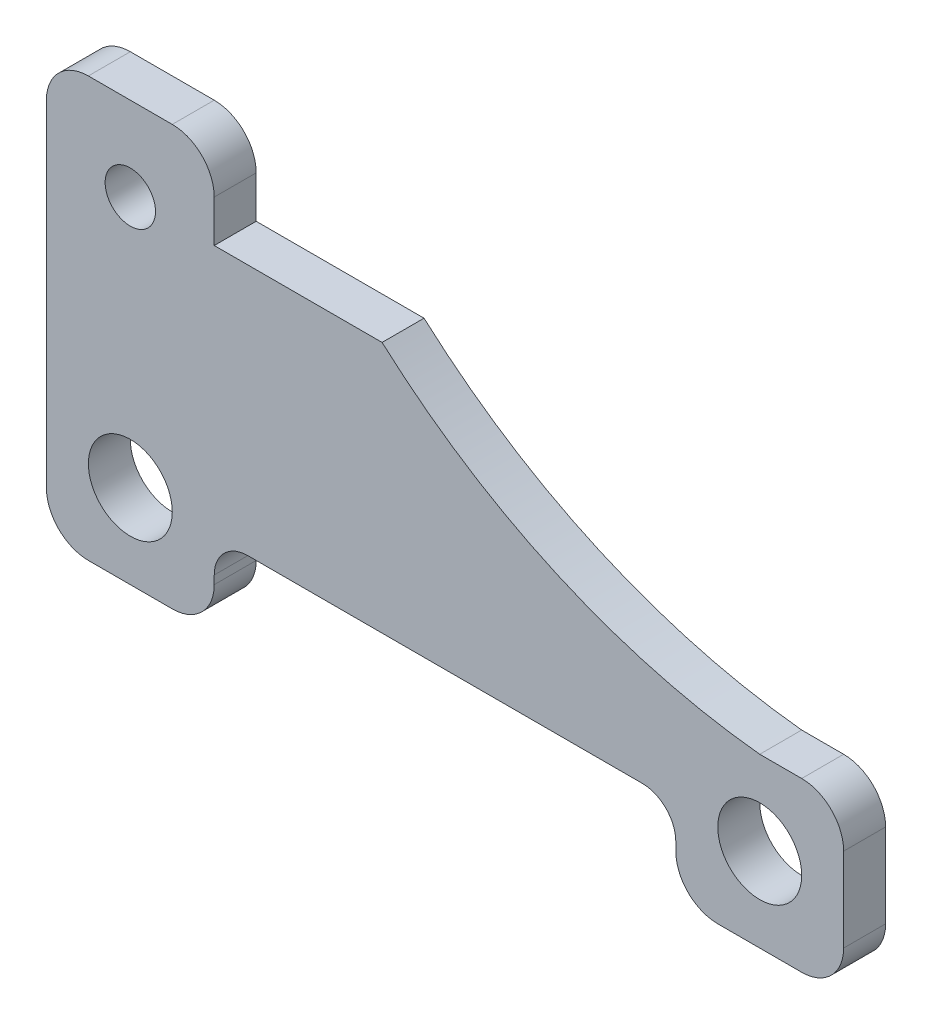
ISO-10303-21;
HEADER;
FILE_DESCRIPTION(('STEP AP214'),'2;1');
FILE_NAME('part.step','',(''),(''),'','','');
FILE_SCHEMA(('AUTOMOTIVE_DESIGN { 1 0 10303 214 1 1 1 1 }'));
ENDSEC;
DATA;
#1=APPLICATION_CONTEXT('core data for automotive mechanical design processes');
#2=APPLICATION_PROTOCOL_DEFINITION('international standard','automotive_design',2000,#1);
#3=PRODUCT_CONTEXT('',#1,'mechanical');
#4=PRODUCT('Part','Part','',(#3));
#5=PRODUCT_RELATED_PRODUCT_CATEGORY('part','',(#4));
#6=PRODUCT_DEFINITION_FORMATION('','',#4);
#7=PRODUCT_DEFINITION_CONTEXT('part definition',#1,'design');
#8=PRODUCT_DEFINITION('design','',#6,#7);
#9=PRODUCT_DEFINITION_SHAPE('','',#8);
#10=(LENGTH_UNIT() NAMED_UNIT(*) SI_UNIT(.MILLI.,.METRE.));
#11=(NAMED_UNIT(*) PLANE_ANGLE_UNIT() SI_UNIT($,.RADIAN.));
#12=(NAMED_UNIT(*) SI_UNIT($,.STERADIAN.) SOLID_ANGLE_UNIT());
#13=UNCERTAINTY_MEASURE_WITH_UNIT(LENGTH_MEASURE(1.E-05),#10,'distance_accuracy_value','');
#14=(GEOMETRIC_REPRESENTATION_CONTEXT(3) GLOBAL_UNCERTAINTY_ASSIGNED_CONTEXT((#13)) GLOBAL_UNIT_ASSIGNED_CONTEXT((#10,
#11,#12)) REPRESENTATION_CONTEXT('',''));
#15=CARTESIAN_POINT('',(0.,0.,0.));
#16=DIRECTION('',(0.,0.,1.));
#17=DIRECTION('',(1.,0.,0.));
#18=AXIS2_PLACEMENT_3D('',#15,#16,#17);
#19=CARTESIAN_POINT('',(80.,-5.,5.));
#20=DIRECTION('',(0.,0.,1.));
#21=DIRECTION('',(1.,0.,0.));
#22=AXIS2_PLACEMENT_3D('',#19,#20,#21);
#23=PLANE('',#22);
#24=CARTESIAN_POINT('',(75.,0.,5.));
#25=DIRECTION('',(0.,0.,1.));
#26=DIRECTION('',(1.,0.,0.));
#27=AXIS2_PLACEMENT_3D('',#24,#25,#26);
#28=CIRCLE('',#27,5.);
#29=CARTESIAN_POINT('',(80.,0.,5.));
#30=VERTEX_POINT('',#29);
#31=EDGE_CURVE('E378',#30,#30,#28,.T.);
#32=ORIENTED_EDGE('',*,*,#31,.F.);
#33=EDGE_LOOP('',(#32));
#34=FACE_BOUND('',#33,.T.);
#35=DIRECTION('',(1.,0.,0.));
#36=VECTOR('',#35,1.);
#37=CARTESIAN_POINT('',(75.,-10.,5.));
#38=LINE('',#37,#36);
#39=CARTESIAN_POINT('',(70.,-10.,5.));
#40=VERTEX_POINT('',#39);
#41=CARTESIAN_POINT('',(80.,-10.,5.));
#42=VERTEX_POINT('',#41);
#43=EDGE_CURVE('E59',#40,#42,#38,.T.);
#44=ORIENTED_EDGE('',*,*,#43,.T.);
#45=CARTESIAN_POINT('',(80.,-5.,5.));
#46=DIRECTION('',(0.,0.,1.));
#47=DIRECTION('',(1.,0.,0.));
#48=AXIS2_PLACEMENT_3D('',#45,#46,#47);
#49=CIRCLE('',#48,5.);
#50=CARTESIAN_POINT('',(85.,-4.99999999999996,5.));
#51=VERTEX_POINT('',#50);
#52=EDGE_CURVE('E143',#42,#51,#49,.T.);
#53=ORIENTED_EDGE('',*,*,#52,.T.);
#54=DIRECTION('',(0.,1.,0.));
#55=VECTOR('',#54,1.);
#56=CARTESIAN_POINT('',(85.,-4.99999999999996,5.));
#57=LINE('',#56,#55);
#58=CARTESIAN_POINT('',(85.,4.99999999999997,5.));
#59=VERTEX_POINT('',#58);
#60=EDGE_CURVE('E311',#51,#59,#57,.T.);
#61=ORIENTED_EDGE('',*,*,#60,.T.);
#62=CARTESIAN_POINT('',(80.,5.,5.));
#63=DIRECTION('',(0.,0.,1.));
#64=DIRECTION('',(1.,0.,0.));
#65=AXIS2_PLACEMENT_3D('',#62,#63,#64);
#66=CIRCLE('',#65,5.);
#67=CARTESIAN_POINT('',(80.,10.,5.));
#68=VERTEX_POINT('',#67);
#69=EDGE_CURVE('E334',#59,#68,#66,.T.);
#70=ORIENTED_EDGE('',*,*,#69,.T.);
#71=DIRECTION('',(-1.,0.,0.));
#72=VECTOR('',#71,1.);
#73=CARTESIAN_POINT('',(80.,10.,5.));
#74=LINE('',#73,#72);
#75=CARTESIAN_POINT('',(75.,9.99999999999998,5.));
#76=VERTEX_POINT('',#75);
#77=EDGE_CURVE('E329',#68,#76,#74,.T.);
#78=ORIENTED_EDGE('',*,*,#77,.T.);
#79=CARTESIAN_POINT('',(83.4139143929199,89.5563073840699,5.));
#80=DIRECTION('',(0.,0.,-1.));
#81=DIRECTION('',(-1.,0.,0.));
#82=AXIS2_PLACEMENT_3D('',#79,#80,#81);
#83=CIRCLE('',#82,80.);
#84=CARTESIAN_POINT('',(30.,30.,5.));
#85=VERTEX_POINT('',#84);
#86=EDGE_CURVE('E335',#76,#85,#83,.T.);
#87=ORIENTED_EDGE('',*,*,#86,.T.);
#88=DIRECTION('',(-1.,0.,0.));
#89=VECTOR('',#88,1.);
#90=CARTESIAN_POINT('',(10.,30.,5.));
#91=LINE('',#90,#89);
#92=CARTESIAN_POINT('',(10.,30.,5.));
#93=VERTEX_POINT('',#92);
#94=EDGE_CURVE('E333',#85,#93,#91,.T.);
#95=ORIENTED_EDGE('',*,*,#94,.T.);
#96=DIRECTION('',(0.,1.,0.));
#97=VECTOR('',#96,1.);
#98=CARTESIAN_POINT('',(10.,35.,5.));
#99=LINE('',#98,#97);
#100=CARTESIAN_POINT('',(10.,35.,5.));
#101=VERTEX_POINT('',#100);
#102=EDGE_CURVE('E341',#93,#101,#99,.T.);
#103=ORIENTED_EDGE('',*,*,#102,.T.);
#104=CARTESIAN_POINT('',(5.,35.,5.));
#105=DIRECTION('',(0.,0.,1.));
#106=DIRECTION('',(-1.,0.,0.));
#107=AXIS2_PLACEMENT_3D('',#104,#105,#106);
#108=CIRCLE('',#107,5.);
#109=CARTESIAN_POINT('',(4.99999999999997,40.,5.));
#110=VERTEX_POINT('',#109);
#111=EDGE_CURVE('E344',#101,#110,#108,.T.);
#112=ORIENTED_EDGE('',*,*,#111,.T.);
#113=DIRECTION('',(-1.,0.,0.));
#114=VECTOR('',#113,1.);
#115=CARTESIAN_POINT('',(-4.99999999999996,40.,5.));
#116=LINE('',#115,#114);
#117=CARTESIAN_POINT('',(-4.99999999999996,40.,5.));
#118=VERTEX_POINT('',#117);
#119=EDGE_CURVE('E345',#110,#118,#116,.T.);
#120=ORIENTED_EDGE('',*,*,#119,.T.);
#121=CARTESIAN_POINT('',(-5.,35.,5.));
#122=DIRECTION('',(0.,0.,1.));
#123=DIRECTION('',(-1.,0.,0.));
#124=AXIS2_PLACEMENT_3D('',#121,#122,#123);
#125=CIRCLE('',#124,5.);
#126=CARTESIAN_POINT('',(-10.,35.,5.));
#127=VERTEX_POINT('',#126);
#128=EDGE_CURVE('E350',#118,#127,#125,.T.);
#129=ORIENTED_EDGE('',*,*,#128,.T.);
#130=DIRECTION('',(0.,-1.,0.));
#131=VECTOR('',#130,1.);
#132=CARTESIAN_POINT('',(-10.,-4.99999999999997,5.));
#133=LINE('',#132,#131);
#134=CARTESIAN_POINT('',(-10.,-4.99999999999997,5.));
#135=VERTEX_POINT('',#134);
#136=EDGE_CURVE('E349',#127,#135,#133,.T.);
#137=ORIENTED_EDGE('',*,*,#136,.T.);
#138=CARTESIAN_POINT('',(-5.,-5.,5.));
#139=DIRECTION('',(0.,0.,1.));
#140=DIRECTION('',(1.,0.,0.));
#141=AXIS2_PLACEMENT_3D('',#138,#139,#140);
#142=CIRCLE('',#141,5.);
#143=CARTESIAN_POINT('',(-4.99999999999996,-10.,5.));
#144=VERTEX_POINT('',#143);
#145=EDGE_CURVE('E352',#135,#144,#142,.T.);
#146=ORIENTED_EDGE('',*,*,#145,.T.);
#147=DIRECTION('',(1.,0.,0.));
#148=VECTOR('',#147,1.);
#149=CARTESIAN_POINT('',(-4.99999999999996,-10.,5.));
#150=LINE('',#149,#148);
#151=CARTESIAN_POINT('',(4.99999999999997,-10.,5.));
#152=VERTEX_POINT('',#151);
#153=EDGE_CURVE('E354',#144,#152,#150,.T.);
#154=ORIENTED_EDGE('',*,*,#153,.T.);
#155=CARTESIAN_POINT('',(5.,-5.,5.));
#156=DIRECTION('',(0.,0.,1.));
#157=DIRECTION('',(1.,0.,0.));
#158=AXIS2_PLACEMENT_3D('',#155,#156,#157);
#159=CIRCLE('',#158,5.);
#160=CARTESIAN_POINT('',(10.,-4.99999999999997,5.));
#161=VERTEX_POINT('',#160);
#162=EDGE_CURVE('E353',#152,#161,#159,.T.);
#163=ORIENTED_EDGE('',*,*,#162,.T.);
#164=DIRECTION('',(0.,1.,0.));
#165=VECTOR('',#164,1.);
#166=CARTESIAN_POINT('',(10.,-4.99999999999997,5.));
#167=LINE('',#166,#165);
#168=CARTESIAN_POINT('',(10.,-4.00000000000003,5.));
#169=VERTEX_POINT('',#168);
#170=EDGE_CURVE('E357',#161,#169,#167,.T.);
#171=ORIENTED_EDGE('',*,*,#170,.T.);
#172=CARTESIAN_POINT('',(14.,-4.,5.));
#173=DIRECTION('',(0.,0.,-1.));
#174=DIRECTION('',(-1.,0.,0.));
#175=AXIS2_PLACEMENT_3D('',#172,#173,#174);
#176=CIRCLE('',#175,4.);
#177=CARTESIAN_POINT('',(14.,0.,5.));
#178=VERTEX_POINT('',#177);
#179=EDGE_CURVE('E358',#169,#178,#176,.T.);
#180=ORIENTED_EDGE('',*,*,#179,.T.);
#181=DIRECTION('',(1.,0.,0.));
#182=VECTOR('',#181,1.);
#183=CARTESIAN_POINT('',(14.,0.,5.));
#184=LINE('',#183,#182);
#185=CARTESIAN_POINT('',(61.,0.,5.));
#186=VERTEX_POINT('',#185);
#187=EDGE_CURVE('E199',#178,#186,#184,.T.);
#188=ORIENTED_EDGE('',*,*,#187,.T.);
#189=CARTESIAN_POINT('',(61.,-4.,5.));
#190=DIRECTION('',(0.,0.,-1.));
#191=DIRECTION('',(-1.,0.,0.));
#192=AXIS2_PLACEMENT_3D('',#189,#190,#191);
#193=CIRCLE('',#192,4.);
#194=CARTESIAN_POINT('',(65.,-4.00000000000003,5.));
#195=VERTEX_POINT('',#194);
#196=EDGE_CURVE('E193',#186,#195,#193,.T.);
#197=ORIENTED_EDGE('',*,*,#196,.T.);
#198=DIRECTION('',(0.,-1.,0.));
#199=VECTOR('',#198,1.);
#200=CARTESIAN_POINT('',(65.,-4.00000000000003,5.));
#201=LINE('',#200,#199);
#202=CARTESIAN_POINT('',(65.,-4.99999999999996,5.));
#203=VERTEX_POINT('',#202);
#204=EDGE_CURVE('E196',#195,#203,#201,.T.);
#205=ORIENTED_EDGE('',*,*,#204,.T.);
#206=CARTESIAN_POINT('',(70.,-5.,5.));
#207=DIRECTION('',(0.,0.,1.));
#208=DIRECTION('',(1.,0.,0.));
#209=AXIS2_PLACEMENT_3D('',#206,#207,#208);
#210=CIRCLE('',#209,5.);
#211=EDGE_CURVE('E212',#203,#40,#210,.T.);
#212=ORIENTED_EDGE('',*,*,#211,.T.);
#213=EDGE_LOOP('',(#44,#53,#61,#70,#78,#87,#95,#103,#112,#120,#129,#137,#146,#154,#163,#171,
#180,#188,#197,#205,#212));
#214=FACE_BOUND('',#213,.T.);
#215=CARTESIAN_POINT('',(0.,0.,5.));
#216=DIRECTION('',(0.,0.,1.));
#217=DIRECTION('',(1.,0.,0.));
#218=AXIS2_PLACEMENT_3D('',#215,#216,#217);
#219=CIRCLE('',#218,5.);
#220=CARTESIAN_POINT('',(5.,0.,5.));
#221=VERTEX_POINT('',#220);
#222=EDGE_CURVE('E224',#221,#221,#219,.T.);
#223=ORIENTED_EDGE('',*,*,#222,.F.);
#224=EDGE_LOOP('',(#223));
#225=FACE_BOUND('',#224,.T.);
#226=CARTESIAN_POINT('',(0.,30.,5.));
#227=DIRECTION('',(0.,0.,1.));
#228=DIRECTION('',(1.,0.,0.));
#229=AXIS2_PLACEMENT_3D('',#226,#227,#228);
#230=CIRCLE('',#229,3.);
#231=CARTESIAN_POINT('',(3.,30.,5.));
#232=VERTEX_POINT('',#231);
#233=EDGE_CURVE('E383',#232,#232,#230,.T.);
#234=ORIENTED_EDGE('',*,*,#233,.F.);
#235=EDGE_LOOP('',(#234));
#236=FACE_BOUND('',#235,.T.);
#237=ADVANCED_FACE('F41',(#34,#214,#225,#236),#23,.T.);
#238=CARTESIAN_POINT('',(80.,-5.,0.));
#239=DIRECTION('',(0.,0.,1.));
#240=DIRECTION('',(1.,0.,0.));
#241=AXIS2_PLACEMENT_3D('',#238,#239,#240);
#242=PLANE('',#241);
#243=CARTESIAN_POINT('',(80.,-5.,0.));
#244=DIRECTION('',(0.,0.,1.));
#245=DIRECTION('',(1.,0.,0.));
#246=AXIS2_PLACEMENT_3D('',#243,#244,#245);
#247=CIRCLE('',#246,5.);
#248=CARTESIAN_POINT('',(80.,-10.,0.));
#249=VERTEX_POINT('',#248);
#250=CARTESIAN_POINT('',(85.,-4.99999999999996,0.));
#251=VERTEX_POINT('',#250);
#252=EDGE_CURVE('E219',#249,#251,#247,.T.);
#253=ORIENTED_EDGE('',*,*,#252,.F.);
#254=DIRECTION('',(1.,0.,0.));
#255=VECTOR('',#254,1.);
#256=CARTESIAN_POINT('',(70.,-10.,0.));
#257=LINE('',#256,#255);
#258=CARTESIAN_POINT('',(70.,-10.,0.));
#259=VERTEX_POINT('',#258);
#260=EDGE_CURVE('E256',#259,#249,#257,.T.);
#261=ORIENTED_EDGE('',*,*,#260,.F.);
#262=CARTESIAN_POINT('',(70.,-5.,0.));
#263=DIRECTION('',(0.,0.,1.));
#264=DIRECTION('',(1.,0.,0.));
#265=AXIS2_PLACEMENT_3D('',#262,#263,#264);
#266=CIRCLE('',#265,5.);
#267=CARTESIAN_POINT('',(65.,-4.99999999999996,0.));
#268=VERTEX_POINT('',#267);
#269=EDGE_CURVE('E131',#268,#259,#266,.T.);
#270=ORIENTED_EDGE('',*,*,#269,.F.);
#271=DIRECTION('',(0.,-1.,0.));
#272=VECTOR('',#271,1.);
#273=CARTESIAN_POINT('',(65.,-4.00000000000003,0.));
#274=LINE('',#273,#272);
#275=CARTESIAN_POINT('',(65.,-4.00000000000003,0.));
#276=VERTEX_POINT('',#275);
#277=EDGE_CURVE('E130',#276,#268,#274,.T.);
#278=ORIENTED_EDGE('',*,*,#277,.F.);
#279=CARTESIAN_POINT('',(61.,-4.,0.));
#280=DIRECTION('',(0.,0.,-1.));
#281=DIRECTION('',(-1.,0.,0.));
#282=AXIS2_PLACEMENT_3D('',#279,#280,#281);
#283=CIRCLE('',#282,4.);
#284=CARTESIAN_POINT('',(61.,0.,0.));
#285=VERTEX_POINT('',#284);
#286=EDGE_CURVE('E208',#285,#276,#283,.T.);
#287=ORIENTED_EDGE('',*,*,#286,.F.);
#288=DIRECTION('',(1.,0.,0.));
#289=VECTOR('',#288,1.);
#290=CARTESIAN_POINT('',(14.,0.,0.));
#291=LINE('',#290,#289);
#292=CARTESIAN_POINT('',(14.,0.,0.));
#293=VERTEX_POINT('',#292);
#294=EDGE_CURVE('E251',#293,#285,#291,.T.);
#295=ORIENTED_EDGE('',*,*,#294,.F.);
#296=CARTESIAN_POINT('',(14.,-4.,0.));
#297=DIRECTION('',(0.,0.,-1.));
#298=DIRECTION('',(-1.,0.,0.));
#299=AXIS2_PLACEMENT_3D('',#296,#297,#298);
#300=CIRCLE('',#299,4.);
#301=CARTESIAN_POINT('',(10.,-4.00000000000003,0.));
#302=VERTEX_POINT('',#301);
#303=EDGE_CURVE('E253',#302,#293,#300,.T.);
#304=ORIENTED_EDGE('',*,*,#303,.F.);
#305=DIRECTION('',(0.,1.,0.));
#306=VECTOR('',#305,1.);
#307=CARTESIAN_POINT('',(10.,-4.99999999999997,0.));
#308=LINE('',#307,#306);
#309=CARTESIAN_POINT('',(10.,-4.99999999999997,0.));
#310=VERTEX_POINT('',#309);
#311=EDGE_CURVE('E248',#310,#302,#308,.T.);
#312=ORIENTED_EDGE('',*,*,#311,.F.);
#313=CARTESIAN_POINT('',(5.,-5.,0.));
#314=DIRECTION('',(0.,0.,1.));
#315=DIRECTION('',(1.,0.,0.));
#316=AXIS2_PLACEMENT_3D('',#313,#314,#315);
#317=CIRCLE('',#316,5.);
#318=CARTESIAN_POINT('',(4.99999999999997,-10.,0.));
#319=VERTEX_POINT('',#318);
#320=EDGE_CURVE('E247',#319,#310,#317,.T.);
#321=ORIENTED_EDGE('',*,*,#320,.F.);
#322=DIRECTION('',(1.,0.,0.));
#323=VECTOR('',#322,1.);
#324=CARTESIAN_POINT('',(-4.99999999999996,-10.,0.));
#325=LINE('',#324,#323);
#326=CARTESIAN_POINT('',(-4.99999999999996,-10.,0.));
#327=VERTEX_POINT('',#326);
#328=EDGE_CURVE('E243',#327,#319,#325,.T.);
#329=ORIENTED_EDGE('',*,*,#328,.F.);
#330=CARTESIAN_POINT('',(-5.,-5.,0.));
#331=DIRECTION('',(0.,0.,1.));
#332=DIRECTION('',(1.,0.,0.));
#333=AXIS2_PLACEMENT_3D('',#330,#331,#332);
#334=CIRCLE('',#333,5.);
#335=CARTESIAN_POINT('',(-10.,-4.99999999999997,0.));
#336=VERTEX_POINT('',#335);
#337=EDGE_CURVE('E244',#336,#327,#334,.T.);
#338=ORIENTED_EDGE('',*,*,#337,.F.);
#339=DIRECTION('',(0.,-1.,0.));
#340=VECTOR('',#339,1.);
#341=CARTESIAN_POINT('',(-10.,-4.99999999999997,0.));
#342=LINE('',#341,#340);
#343=CARTESIAN_POINT('',(-10.,35.,0.));
#344=VERTEX_POINT('',#343);
#345=EDGE_CURVE('E242',#344,#336,#342,.T.);
#346=ORIENTED_EDGE('',*,*,#345,.F.);
#347=CARTESIAN_POINT('',(-5.,35.,0.));
#348=DIRECTION('',(0.,0.,1.));
#349=DIRECTION('',(-1.,0.,0.));
#350=AXIS2_PLACEMENT_3D('',#347,#348,#349);
#351=CIRCLE('',#350,5.);
#352=CARTESIAN_POINT('',(-4.99999999999996,40.,0.));
#353=VERTEX_POINT('',#352);
#354=EDGE_CURVE('E239',#353,#344,#351,.T.);
#355=ORIENTED_EDGE('',*,*,#354,.F.);
#356=DIRECTION('',(-1.,0.,0.));
#357=VECTOR('',#356,1.);
#358=CARTESIAN_POINT('',(-4.99999999999996,40.,0.));
#359=LINE('',#358,#357);
#360=CARTESIAN_POINT('',(4.99999999999997,40.,0.));
#361=VERTEX_POINT('',#360);
#362=EDGE_CURVE('E240',#361,#353,#359,.T.);
#363=ORIENTED_EDGE('',*,*,#362,.F.);
#364=CARTESIAN_POINT('',(5.,35.,0.));
#365=DIRECTION('',(0.,0.,1.));
#366=DIRECTION('',(-1.,0.,0.));
#367=AXIS2_PLACEMENT_3D('',#364,#365,#366);
#368=CIRCLE('',#367,5.);
#369=CARTESIAN_POINT('',(10.,35.,0.));
#370=VERTEX_POINT('',#369);
#371=EDGE_CURVE('E235',#370,#361,#368,.T.);
#372=ORIENTED_EDGE('',*,*,#371,.F.);
#373=DIRECTION('',(0.,1.,0.));
#374=VECTOR('',#373,1.);
#375=CARTESIAN_POINT('',(10.,35.,0.));
#376=LINE('',#375,#374);
#377=CARTESIAN_POINT('',(10.,30.,0.));
#378=VERTEX_POINT('',#377);
#379=EDGE_CURVE('E234',#378,#370,#376,.T.);
#380=ORIENTED_EDGE('',*,*,#379,.F.);
#381=DIRECTION('',(-1.,0.,0.));
#382=VECTOR('',#381,1.);
#383=CARTESIAN_POINT('',(10.,30.,0.));
#384=LINE('',#383,#382);
#385=CARTESIAN_POINT('',(30.,30.,0.));
#386=VERTEX_POINT('',#385);
#387=EDGE_CURVE('E231',#386,#378,#384,.T.);
#388=ORIENTED_EDGE('',*,*,#387,.F.);
#389=CARTESIAN_POINT('',(83.4139143929199,89.5563073840699,0.));
#390=DIRECTION('',(0.,0.,-1.));
#391=DIRECTION('',(-1.,0.,0.));
#392=AXIS2_PLACEMENT_3D('',#389,#390,#391);
#393=CIRCLE('',#392,80.);
#394=CARTESIAN_POINT('',(75.,9.99999999999998,0.));
#395=VERTEX_POINT('',#394);
#396=EDGE_CURVE('E226',#395,#386,#393,.T.);
#397=ORIENTED_EDGE('',*,*,#396,.F.);
#398=DIRECTION('',(-1.,0.,0.));
#399=VECTOR('',#398,1.);
#400=CARTESIAN_POINT('',(80.,10.,0.));
#401=LINE('',#400,#399);
#402=CARTESIAN_POINT('',(80.,10.,0.));
#403=VERTEX_POINT('',#402);
#404=EDGE_CURVE('E230',#403,#395,#401,.T.);
#405=ORIENTED_EDGE('',*,*,#404,.F.);
#406=CARTESIAN_POINT('',(80.,5.,0.));
#407=DIRECTION('',(0.,0.,1.));
#408=DIRECTION('',(1.,0.,0.));
#409=AXIS2_PLACEMENT_3D('',#406,#407,#408);
#410=CIRCLE('',#409,5.);
#411=CARTESIAN_POINT('',(85.,4.99999999999997,0.));
#412=VERTEX_POINT('',#411);
#413=EDGE_CURVE('E223',#412,#403,#410,.T.);
#414=ORIENTED_EDGE('',*,*,#413,.F.);
#415=DIRECTION('',(0.,1.,0.));
#416=VECTOR('',#415,1.);
#417=CARTESIAN_POINT('',(85.,-4.99999999999996,0.));
#418=LINE('',#417,#416);
#419=EDGE_CURVE('E225',#251,#412,#418,.T.);
#420=ORIENTED_EDGE('',*,*,#419,.F.);
#421=EDGE_LOOP('',(#253,#261,#270,#278,#287,#295,#304,#312,#321,#329,#338,#346,#355,#363,#372,
#380,#388,#397,#405,#414,#420));
#422=FACE_BOUND('',#421,.T.);
#423=CARTESIAN_POINT('',(0.,0.,0.));
#424=DIRECTION('',(0.,0.,1.));
#425=DIRECTION('',(1.,0.,0.));
#426=AXIS2_PLACEMENT_3D('',#423,#424,#425);
#427=CIRCLE('',#426,5.);
#428=CARTESIAN_POINT('',(5.,0.,0.));
#429=VERTEX_POINT('',#428);
#430=EDGE_CURVE('E374',#429,#429,#427,.T.);
#431=ORIENTED_EDGE('',*,*,#430,.T.);
#432=EDGE_LOOP('',(#431));
#433=FACE_BOUND('',#432,.T.);
#434=CARTESIAN_POINT('',(75.,0.,0.));
#435=DIRECTION('',(0.,0.,1.));
#436=DIRECTION('',(1.,0.,0.));
#437=AXIS2_PLACEMENT_3D('',#434,#435,#436);
#438=CIRCLE('',#437,5.);
#439=CARTESIAN_POINT('',(80.,0.,0.));
#440=VERTEX_POINT('',#439);
#441=EDGE_CURVE('E381',#440,#440,#438,.T.);
#442=ORIENTED_EDGE('',*,*,#441,.T.);
#443=EDGE_LOOP('',(#442));
#444=FACE_BOUND('',#443,.T.);
#445=CARTESIAN_POINT('',(0.,30.,0.));
#446=DIRECTION('',(0.,0.,1.));
#447=DIRECTION('',(1.,0.,0.));
#448=AXIS2_PLACEMENT_3D('',#445,#446,#447);
#449=CIRCLE('',#448,3.);
#450=CARTESIAN_POINT('',(3.,30.,0.));
#451=VERTEX_POINT('',#450);
#452=EDGE_CURVE('E390',#451,#451,#449,.T.);
#453=ORIENTED_EDGE('',*,*,#452,.T.);
#454=EDGE_LOOP('',(#453));
#455=FACE_BOUND('',#454,.T.);
#456=ADVANCED_FACE('F320',(#422,#433,#444,#455),#242,.F.);
#457=CARTESIAN_POINT('',(80.,-5.,5.));
#458=DIRECTION('',(0.,0.,-1.));
#459=DIRECTION('',(-1.,0.,0.));
#460=AXIS2_PLACEMENT_3D('',#457,#458,#459);
#461=CYLINDRICAL_SURFACE('',#460,5.);
#462=ORIENTED_EDGE('',*,*,#252,.T.);
#463=DIRECTION('',(0.,0.,-1.));
#464=VECTOR('',#463,1.);
#465=CARTESIAN_POINT('',(85.,-4.99999999999996,5.));
#466=LINE('',#465,#464);
#467=EDGE_CURVE('E49',#51,#251,#466,.T.);
#468=ORIENTED_EDGE('',*,*,#467,.F.);
#469=ORIENTED_EDGE('',*,*,#52,.F.);
#470=DIRECTION('',(0.,0.,-1.));
#471=VECTOR('',#470,1.);
#472=CARTESIAN_POINT('',(80.,-10.,5.));
#473=LINE('',#472,#471);
#474=EDGE_CURVE('E11',#42,#249,#473,.T.);
#475=ORIENTED_EDGE('',*,*,#474,.T.);
#476=EDGE_LOOP('',(#462,#468,#469,#475));
#477=FACE_BOUND('',#476,.T.);
#478=ADVANCED_FACE('F43',(#477),#461,.T.);
#479=CARTESIAN_POINT('',(85.,-4.99999999999996,5.));
#480=DIRECTION('',(-1.,0.,0.));
#481=DIRECTION('',(0.,0.,1.));
#482=AXIS2_PLACEMENT_3D('',#479,#480,#481);
#483=PLANE('',#482);
#484=ORIENTED_EDGE('',*,*,#419,.T.);
#485=DIRECTION('',(0.,0.,-1.));
#486=VECTOR('',#485,1.);
#487=CARTESIAN_POINT('',(85.,4.99999999999997,5.));
#488=LINE('',#487,#486);
#489=EDGE_CURVE('E305',#59,#412,#488,.T.);
#490=ORIENTED_EDGE('',*,*,#489,.F.);
#491=ORIENTED_EDGE('',*,*,#60,.F.);
#492=ORIENTED_EDGE('',*,*,#467,.T.);
#493=EDGE_LOOP('',(#484,#490,#491,#492));
#494=FACE_BOUND('',#493,.T.);
#495=ADVANCED_FACE('F313',(#494),#483,.F.);
#496=CARTESIAN_POINT('',(80.,5.,5.));
#497=DIRECTION('',(0.,0.,-1.));
#498=DIRECTION('',(-1.,0.,0.));
#499=AXIS2_PLACEMENT_3D('',#496,#497,#498);
#500=CYLINDRICAL_SURFACE('',#499,5.);
#501=ORIENTED_EDGE('',*,*,#413,.T.);
#502=DIRECTION('',(0.,0.,-1.));
#503=VECTOR('',#502,1.);
#504=CARTESIAN_POINT('',(80.,10.,5.));
#505=LINE('',#504,#503);
#506=EDGE_CURVE('E302',#68,#403,#505,.T.);
#507=ORIENTED_EDGE('',*,*,#506,.F.);
#508=ORIENTED_EDGE('',*,*,#69,.F.);
#509=ORIENTED_EDGE('',*,*,#489,.T.);
#510=EDGE_LOOP('',(#501,#507,#508,#509));
#511=FACE_BOUND('',#510,.T.);
#512=ADVANCED_FACE('F322',(#511),#500,.T.);
#513=CARTESIAN_POINT('',(80.,10.,5.));
#514=DIRECTION('',(0.,-1.,0.));
#515=DIRECTION('',(0.,0.,-1.));
#516=AXIS2_PLACEMENT_3D('',#513,#514,#515);
#517=PLANE('',#516);
#518=ORIENTED_EDGE('',*,*,#404,.T.);
#519=DIRECTION('',(0.,0.,-1.));
#520=VECTOR('',#519,1.);
#521=CARTESIAN_POINT('',(75.,9.99999999999998,5.));
#522=LINE('',#521,#520);
#523=EDGE_CURVE('E296',#76,#395,#522,.T.);
#524=ORIENTED_EDGE('',*,*,#523,.F.);
#525=ORIENTED_EDGE('',*,*,#77,.F.);
#526=ORIENTED_EDGE('',*,*,#506,.T.);
#527=EDGE_LOOP('',(#518,#524,#525,#526));
#528=FACE_BOUND('',#527,.T.);
#529=ADVANCED_FACE('F327',(#528),#517,.F.);
#530=CARTESIAN_POINT('',(83.4139143929199,89.5563073840699,5.));
#531=DIRECTION('',(0.,0.,-1.));
#532=DIRECTION('',(-1.,0.,0.));
#533=AXIS2_PLACEMENT_3D('',#530,#531,#532);
#534=CYLINDRICAL_SURFACE('',#533,80.);
#535=ORIENTED_EDGE('',*,*,#396,.T.);
#536=DIRECTION('',(0.,0.,-1.));
#537=VECTOR('',#536,1.);
#538=CARTESIAN_POINT('',(30.,30.,5.));
#539=LINE('',#538,#537);
#540=EDGE_CURVE('E297',#85,#386,#539,.T.);
#541=ORIENTED_EDGE('',*,*,#540,.F.);
#542=ORIENTED_EDGE('',*,*,#86,.F.);
#543=ORIENTED_EDGE('',*,*,#523,.T.);
#544=EDGE_LOOP('',(#535,#541,#542,#543));
#545=FACE_BOUND('',#544,.T.);
#546=ADVANCED_FACE('F459',(#545),#534,.F.);
#547=CARTESIAN_POINT('',(10.,30.,5.));
#548=DIRECTION('',(0.,-1.,0.));
#549=DIRECTION('',(0.,0.,-1.));
#550=AXIS2_PLACEMENT_3D('',#547,#548,#549);
#551=PLANE('',#550);
#552=ORIENTED_EDGE('',*,*,#387,.T.);
#553=DIRECTION('',(0.,0.,-1.));
#554=VECTOR('',#553,1.);
#555=CARTESIAN_POINT('',(10.,30.,5.));
#556=LINE('',#555,#554);
#557=EDGE_CURVE('E291',#93,#378,#556,.T.);
#558=ORIENTED_EDGE('',*,*,#557,.F.);
#559=ORIENTED_EDGE('',*,*,#94,.F.);
#560=ORIENTED_EDGE('',*,*,#540,.T.);
#561=EDGE_LOOP('',(#552,#558,#559,#560));
#562=FACE_BOUND('',#561,.T.);
#563=ADVANCED_FACE('F455',(#562),#551,.F.);
#564=CARTESIAN_POINT('',(10.,35.,5.));
#565=DIRECTION('',(-1.,0.,0.));
#566=DIRECTION('',(0.,0.,1.));
#567=AXIS2_PLACEMENT_3D('',#564,#565,#566);
#568=PLANE('',#567);
#569=ORIENTED_EDGE('',*,*,#379,.T.);
#570=DIRECTION('',(0.,0.,-1.));
#571=VECTOR('',#570,1.);
#572=CARTESIAN_POINT('',(10.,35.,5.));
#573=LINE('',#572,#571);
#574=EDGE_CURVE('E290',#101,#370,#573,.T.);
#575=ORIENTED_EDGE('',*,*,#574,.F.);
#576=ORIENTED_EDGE('',*,*,#102,.F.);
#577=ORIENTED_EDGE('',*,*,#557,.T.);
#578=EDGE_LOOP('',(#569,#575,#576,#577));
#579=FACE_BOUND('',#578,.T.);
#580=ADVANCED_FACE('F451',(#579),#568,.F.);
#581=CARTESIAN_POINT('',(5.,35.,5.));
#582=DIRECTION('',(0.,0.,-1.));
#583=DIRECTION('',(-1.,0.,0.));
#584=AXIS2_PLACEMENT_3D('',#581,#582,#583);
#585=CYLINDRICAL_SURFACE('',#584,5.);
#586=ORIENTED_EDGE('',*,*,#371,.T.);
#587=DIRECTION('',(0.,0.,-1.));
#588=VECTOR('',#587,1.);
#589=CARTESIAN_POINT('',(4.99999999999997,40.,5.));
#590=LINE('',#589,#588);
#591=EDGE_CURVE('E287',#110,#361,#590,.T.);
#592=ORIENTED_EDGE('',*,*,#591,.F.);
#593=ORIENTED_EDGE('',*,*,#111,.F.);
#594=ORIENTED_EDGE('',*,*,#574,.T.);
#595=EDGE_LOOP('',(#586,#592,#593,#594));
#596=FACE_BOUND('',#595,.T.);
#597=ADVANCED_FACE('F450',(#596),#585,.T.);
#598=CARTESIAN_POINT('',(-4.99999999999996,40.,5.));
#599=DIRECTION('',(0.,-1.,0.));
#600=DIRECTION('',(0.,0.,-1.));
#601=AXIS2_PLACEMENT_3D('',#598,#599,#600);
#602=PLANE('',#601);
#603=ORIENTED_EDGE('',*,*,#362,.T.);
#604=DIRECTION('',(0.,0.,-1.));
#605=VECTOR('',#604,1.);
#606=CARTESIAN_POINT('',(-4.99999999999996,40.,5.));
#607=LINE('',#606,#605);
#608=EDGE_CURVE('E281',#118,#353,#607,.T.);
#609=ORIENTED_EDGE('',*,*,#608,.F.);
#610=ORIENTED_EDGE('',*,*,#119,.F.);
#611=ORIENTED_EDGE('',*,*,#591,.T.);
#612=EDGE_LOOP('',(#603,#609,#610,#611));
#613=FACE_BOUND('',#612,.T.);
#614=ADVANCED_FACE('F444',(#613),#602,.F.);
#615=CARTESIAN_POINT('',(-5.,35.,5.));
#616=DIRECTION('',(0.,0.,-1.));
#617=DIRECTION('',(-1.,0.,0.));
#618=AXIS2_PLACEMENT_3D('',#615,#616,#617);
#619=CYLINDRICAL_SURFACE('',#618,5.);
#620=ORIENTED_EDGE('',*,*,#354,.T.);
#621=DIRECTION('',(0.,0.,-1.));
#622=VECTOR('',#621,1.);
#623=CARTESIAN_POINT('',(-10.,35.,5.));
#624=LINE('',#623,#622);
#625=EDGE_CURVE('E282',#127,#344,#624,.T.);
#626=ORIENTED_EDGE('',*,*,#625,.F.);
#627=ORIENTED_EDGE('',*,*,#128,.F.);
#628=ORIENTED_EDGE('',*,*,#608,.T.);
#629=EDGE_LOOP('',(#620,#626,#627,#628));
#630=FACE_BOUND('',#629,.T.);
#631=ADVANCED_FACE('F438',(#630),#619,.T.);
#632=CARTESIAN_POINT('',(-10.,-4.99999999999997,5.));
#633=DIRECTION('',(1.,0.,0.));
#634=DIRECTION('',(0.,0.,-1.));
#635=AXIS2_PLACEMENT_3D('',#632,#633,#634);
#636=PLANE('',#635);
#637=ORIENTED_EDGE('',*,*,#345,.T.);
#638=DIRECTION('',(0.,0.,-1.));
#639=VECTOR('',#638,1.);
#640=CARTESIAN_POINT('',(-10.,-4.99999999999997,5.));
#641=LINE('',#640,#639);
#642=EDGE_CURVE('E279',#135,#336,#641,.T.);
#643=ORIENTED_EDGE('',*,*,#642,.F.);
#644=ORIENTED_EDGE('',*,*,#136,.F.);
#645=ORIENTED_EDGE('',*,*,#625,.T.);
#646=EDGE_LOOP('',(#637,#643,#644,#645));
#647=FACE_BOUND('',#646,.T.);
#648=ADVANCED_FACE('F434',(#647),#636,.F.);
#649=CARTESIAN_POINT('',(-5.,-5.,5.));
#650=DIRECTION('',(0.,0.,-1.));
#651=DIRECTION('',(-1.,0.,0.));
#652=AXIS2_PLACEMENT_3D('',#649,#650,#651);
#653=CYLINDRICAL_SURFACE('',#652,5.);
#654=ORIENTED_EDGE('',*,*,#337,.T.);
#655=DIRECTION('',(0.,0.,-1.));
#656=VECTOR('',#655,1.);
#657=CARTESIAN_POINT('',(-4.99999999999996,-10.,5.));
#658=LINE('',#657,#656);
#659=EDGE_CURVE('E274',#144,#327,#658,.T.);
#660=ORIENTED_EDGE('',*,*,#659,.F.);
#661=ORIENTED_EDGE('',*,*,#145,.F.);
#662=ORIENTED_EDGE('',*,*,#642,.T.);
#663=EDGE_LOOP('',(#654,#660,#661,#662));
#664=FACE_BOUND('',#663,.T.);
#665=ADVANCED_FACE('F431',(#664),#653,.T.);
#666=CARTESIAN_POINT('',(-4.99999999999996,-10.,5.));
#667=DIRECTION('',(0.,1.,0.));
#668=DIRECTION('',(0.,0.,1.));
#669=AXIS2_PLACEMENT_3D('',#666,#667,#668);
#670=PLANE('',#669);
#671=ORIENTED_EDGE('',*,*,#328,.T.);
#672=DIRECTION('',(0.,0.,-1.));
#673=VECTOR('',#672,1.);
#674=CARTESIAN_POINT('',(4.99999999999997,-10.,5.));
#675=LINE('',#674,#673);
#676=EDGE_CURVE('E275',#152,#319,#675,.T.);
#677=ORIENTED_EDGE('',*,*,#676,.F.);
#678=ORIENTED_EDGE('',*,*,#153,.F.);
#679=ORIENTED_EDGE('',*,*,#659,.T.);
#680=EDGE_LOOP('',(#671,#677,#678,#679));
#681=FACE_BOUND('',#680,.T.);
#682=ADVANCED_FACE('F430',(#681),#670,.F.);
#683=CARTESIAN_POINT('',(5.,-5.,5.));
#684=DIRECTION('',(0.,0.,-1.));
#685=DIRECTION('',(-1.,0.,0.));
#686=AXIS2_PLACEMENT_3D('',#683,#684,#685);
#687=CYLINDRICAL_SURFACE('',#686,5.);
#688=ORIENTED_EDGE('',*,*,#320,.T.);
#689=DIRECTION('',(0.,0.,-1.));
#690=VECTOR('',#689,1.);
#691=CARTESIAN_POINT('',(10.,-4.99999999999997,5.));
#692=LINE('',#691,#690);
#693=EDGE_CURVE('E267',#161,#310,#692,.T.);
#694=ORIENTED_EDGE('',*,*,#693,.F.);
#695=ORIENTED_EDGE('',*,*,#162,.F.);
#696=ORIENTED_EDGE('',*,*,#676,.T.);
#697=EDGE_LOOP('',(#688,#694,#695,#696));
#698=FACE_BOUND('',#697,.T.);
#699=ADVANCED_FACE('F421',(#698),#687,.T.);
#700=CARTESIAN_POINT('',(10.,-4.99999999999997,5.));
#701=DIRECTION('',(-1.,0.,0.));
#702=DIRECTION('',(0.,0.,1.));
#703=AXIS2_PLACEMENT_3D('',#700,#701,#702);
#704=PLANE('',#703);
#705=ORIENTED_EDGE('',*,*,#311,.T.);
#706=DIRECTION('',(0.,0.,-1.));
#707=VECTOR('',#706,1.);
#708=CARTESIAN_POINT('',(10.,-4.00000000000003,5.));
#709=LINE('',#708,#707);
#710=EDGE_CURVE('E266',#169,#302,#709,.T.);
#711=ORIENTED_EDGE('',*,*,#710,.F.);
#712=ORIENTED_EDGE('',*,*,#170,.F.);
#713=ORIENTED_EDGE('',*,*,#693,.T.);
#714=EDGE_LOOP('',(#705,#711,#712,#713));
#715=FACE_BOUND('',#714,.T.);
#716=ADVANCED_FACE('F419',(#715),#704,.F.);
#717=CARTESIAN_POINT('',(14.,-4.,5.));
#718=DIRECTION('',(0.,0.,-1.));
#719=DIRECTION('',(-1.,0.,0.));
#720=AXIS2_PLACEMENT_3D('',#717,#718,#719);
#721=CYLINDRICAL_SURFACE('',#720,4.);
#722=ORIENTED_EDGE('',*,*,#303,.T.);
#723=DIRECTION('',(0.,0.,-1.));
#724=VECTOR('',#723,1.);
#725=CARTESIAN_POINT('',(14.,0.,5.));
#726=LINE('',#725,#724);
#727=EDGE_CURVE('E263',#178,#293,#726,.T.);
#728=ORIENTED_EDGE('',*,*,#727,.F.);
#729=ORIENTED_EDGE('',*,*,#179,.F.);
#730=ORIENTED_EDGE('',*,*,#710,.T.);
#731=EDGE_LOOP('',(#722,#728,#729,#730));
#732=FACE_BOUND('',#731,.T.);
#733=ADVANCED_FACE('F364',(#732),#721,.F.);
#734=CARTESIAN_POINT('',(14.,0.,5.));
#735=DIRECTION('',(0.,1.,0.));
#736=DIRECTION('',(0.,0.,1.));
#737=AXIS2_PLACEMENT_3D('',#734,#735,#736);
#738=PLANE('',#737);
#739=ORIENTED_EDGE('',*,*,#294,.T.);
#740=DIRECTION('',(0.,0.,-1.));
#741=VECTOR('',#740,1.);
#742=CARTESIAN_POINT('',(61.,0.,5.));
#743=LINE('',#742,#741);
#744=EDGE_CURVE('E207',#186,#285,#743,.T.);
#745=ORIENTED_EDGE('',*,*,#744,.F.);
#746=ORIENTED_EDGE('',*,*,#187,.F.);
#747=ORIENTED_EDGE('',*,*,#727,.T.);
#748=EDGE_LOOP('',(#739,#745,#746,#747));
#749=FACE_BOUND('',#748,.T.);
#750=ADVANCED_FACE('F369',(#749),#738,.F.);
#751=CARTESIAN_POINT('',(61.,-4.,5.));
#752=DIRECTION('',(0.,0.,-1.));
#753=DIRECTION('',(-1.,0.,0.));
#754=AXIS2_PLACEMENT_3D('',#751,#752,#753);
#755=CYLINDRICAL_SURFACE('',#754,4.);
#756=ORIENTED_EDGE('',*,*,#286,.T.);
#757=DIRECTION('',(0.,0.,-1.));
#758=VECTOR('',#757,1.);
#759=CARTESIAN_POINT('',(65.,-4.00000000000003,5.));
#760=LINE('',#759,#758);
#761=EDGE_CURVE('E202',#195,#276,#760,.T.);
#762=ORIENTED_EDGE('',*,*,#761,.F.);
#763=ORIENTED_EDGE('',*,*,#196,.F.);
#764=ORIENTED_EDGE('',*,*,#744,.T.);
#765=EDGE_LOOP('',(#756,#762,#763,#764));
#766=FACE_BOUND('',#765,.T.);
#767=ADVANCED_FACE('F206',(#766),#755,.F.);
#768=CARTESIAN_POINT('',(65.,-4.00000000000003,5.));
#769=DIRECTION('',(1.,0.,0.));
#770=DIRECTION('',(0.,0.,-1.));
#771=AXIS2_PLACEMENT_3D('',#768,#769,#770);
#772=PLANE('',#771);
#773=ORIENTED_EDGE('',*,*,#277,.T.);
#774=DIRECTION('',(0.,0.,-1.));
#775=VECTOR('',#774,1.);
#776=CARTESIAN_POINT('',(65.,-4.99999999999996,5.));
#777=LINE('',#776,#775);
#778=EDGE_CURVE('E209',#203,#268,#777,.T.);
#779=ORIENTED_EDGE('',*,*,#778,.F.);
#780=ORIENTED_EDGE('',*,*,#204,.F.);
#781=ORIENTED_EDGE('',*,*,#761,.T.);
#782=EDGE_LOOP('',(#773,#779,#780,#781));
#783=FACE_BOUND('',#782,.T.);
#784=ADVANCED_FACE('F215',(#783),#772,.F.);
#785=CARTESIAN_POINT('',(70.,-5.,5.));
#786=DIRECTION('',(0.,0.,-1.));
#787=DIRECTION('',(-1.,0.,0.));
#788=AXIS2_PLACEMENT_3D('',#785,#786,#787);
#789=CYLINDRICAL_SURFACE('',#788,5.);
#790=ORIENTED_EDGE('',*,*,#269,.T.);
#791=DIRECTION('',(0.,0.,-1.));
#792=VECTOR('',#791,1.);
#793=CARTESIAN_POINT('',(70.,-10.,5.));
#794=LINE('',#793,#792);
#795=EDGE_CURVE('E216',#40,#259,#794,.T.);
#796=ORIENTED_EDGE('',*,*,#795,.F.);
#797=ORIENTED_EDGE('',*,*,#211,.F.);
#798=ORIENTED_EDGE('',*,*,#778,.T.);
#799=EDGE_LOOP('',(#790,#796,#797,#798));
#800=FACE_BOUND('',#799,.T.);
#801=ADVANCED_FACE('F371',(#800),#789,.T.);
#802=CARTESIAN_POINT('',(70.,-10.,5.));
#803=DIRECTION('',(0.,1.,0.));
#804=DIRECTION('',(0.,0.,1.));
#805=AXIS2_PLACEMENT_3D('',#802,#803,#804);
#806=PLANE('',#805);
#807=ORIENTED_EDGE('',*,*,#260,.T.);
#808=ORIENTED_EDGE('',*,*,#474,.F.);
#809=ORIENTED_EDGE('',*,*,#43,.F.);
#810=ORIENTED_EDGE('',*,*,#795,.T.);
#811=EDGE_LOOP('',(#807,#808,#809,#810));
#812=FACE_BOUND('',#811,.T.);
#813=ADVANCED_FACE('F367',(#812),#806,.F.);
#814=CARTESIAN_POINT('',(0.,0.,5.));
#815=DIRECTION('',(0.,0.,-1.));
#816=DIRECTION('',(-1.,0.,0.));
#817=AXIS2_PLACEMENT_3D('',#814,#815,#816);
#818=CYLINDRICAL_SURFACE('',#817,5.);
#819=ORIENTED_EDGE('',*,*,#222,.T.);
#820=EDGE_LOOP('',(#819));
#821=FACE_BOUND('',#820,.T.);
#822=ORIENTED_EDGE('',*,*,#430,.F.);
#823=EDGE_LOOP('',(#822));
#824=FACE_BOUND('',#823,.T.);
#825=ADVANCED_FACE('F403',(#821,#824),#818,.F.);
#826=CARTESIAN_POINT('',(75.,0.,5.));
#827=DIRECTION('',(0.,0.,-1.));
#828=DIRECTION('',(-1.,0.,0.));
#829=AXIS2_PLACEMENT_3D('',#826,#827,#828);
#830=CYLINDRICAL_SURFACE('',#829,5.);
#831=ORIENTED_EDGE('',*,*,#31,.T.);
#832=EDGE_LOOP('',(#831));
#833=FACE_BOUND('',#832,.T.);
#834=ORIENTED_EDGE('',*,*,#441,.F.);
#835=EDGE_LOOP('',(#834));
#836=FACE_BOUND('',#835,.T.);
#837=ADVANCED_FACE('F595',(#833,#836),#830,.F.);
#838=CARTESIAN_POINT('',(0.,30.,5.));
#839=DIRECTION('',(0.,0.,-1.));
#840=DIRECTION('',(-1.,0.,0.));
#841=AXIS2_PLACEMENT_3D('',#838,#839,#840);
#842=CYLINDRICAL_SURFACE('',#841,3.);
#843=ORIENTED_EDGE('',*,*,#233,.T.);
#844=EDGE_LOOP('',(#843));
#845=FACE_BOUND('',#844,.T.);
#846=ORIENTED_EDGE('',*,*,#452,.F.);
#847=EDGE_LOOP('',(#846));
#848=FACE_BOUND('',#847,.T.);
#849=ADVANCED_FACE('F394',(#845,#848),#842,.F.);
#850=CLOSED_SHELL('',(#237,#456,#478,#495,#512,#529,#546,#563,#580,#597,#614,#631,#648,#665,
#682,#699,#716,#733,#750,#767,#784,#801,#813,#825,#837,#849));
#851=MANIFOLD_SOLID_BREP('B2',#850);
#852=ADVANCED_BREP_SHAPE_REPRESENTATION('',(#18,#851),#14);
#853=SHAPE_DEFINITION_REPRESENTATION(#9,#852);
ENDSEC;
END-ISO-10303-21;
